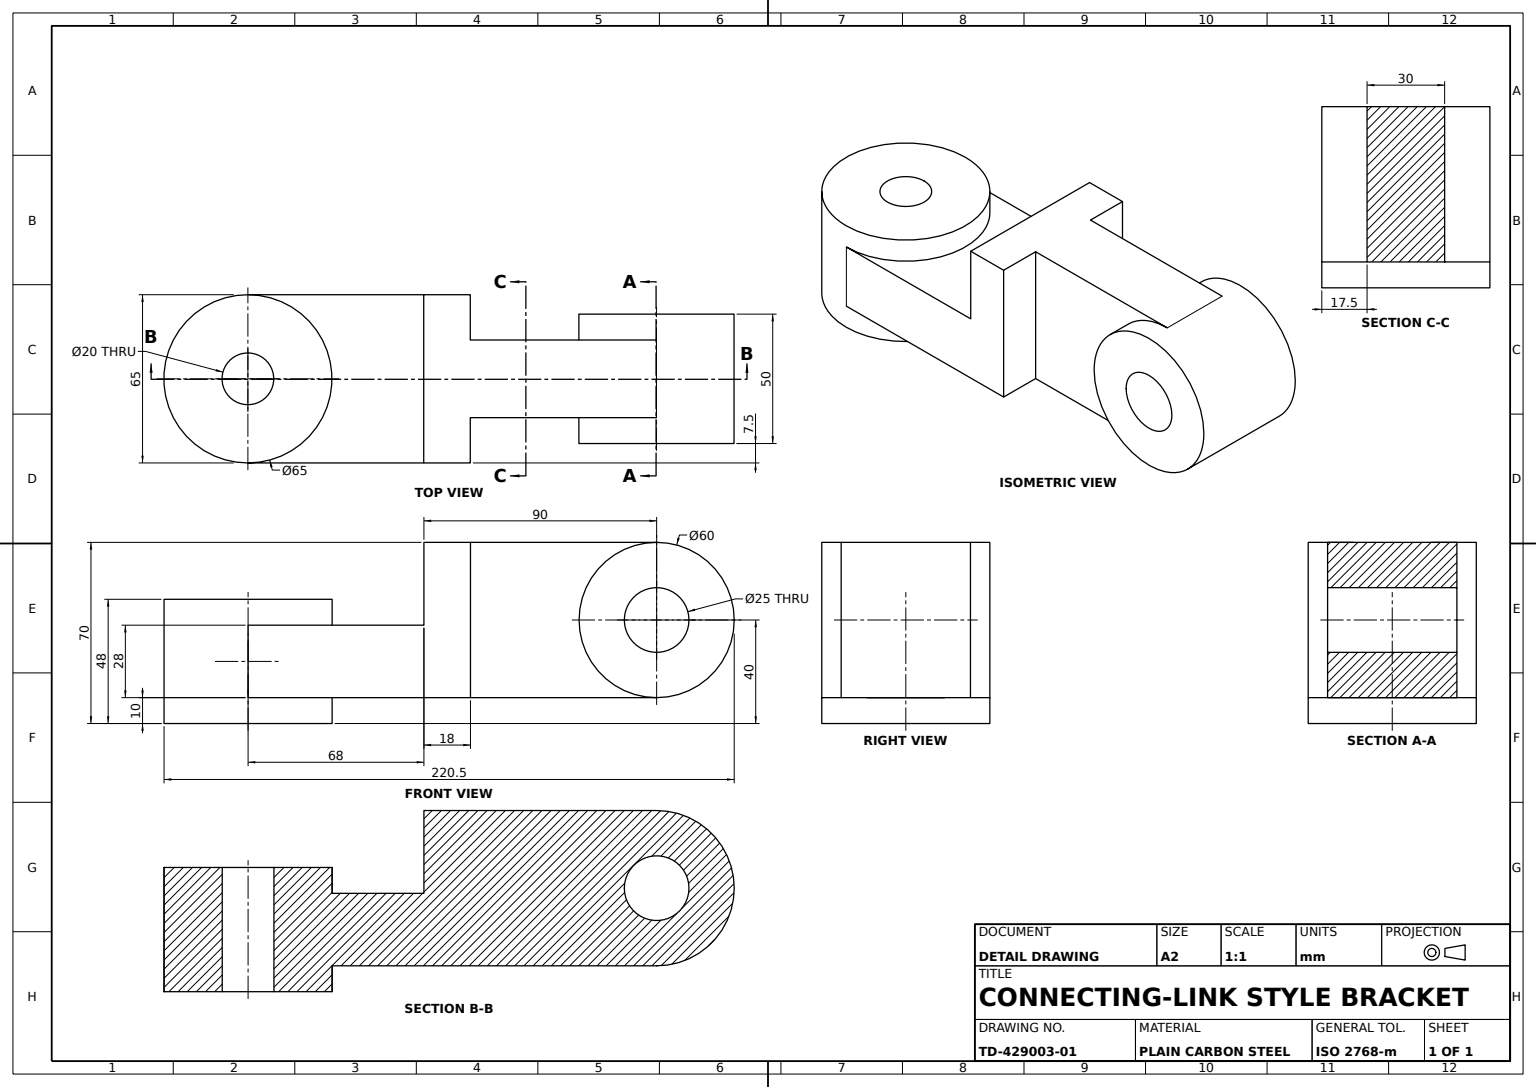
from build123d import *

# Parameters (mm, degrees)
MAIN_BODY_DEPTH                 = 65
CENTER_PAD_SKETCH_W             = 65
CENTER_PAD_SKETCH_H             = 28
CENTER_PAD_DEPTH                = 18
VERTICAL_BOSS_SKETCH_R          = 32.5
VERTICAL_BOSS_DEPTH             = 48
VERTICAL_START                  = 10
VERTICAL_BOSS_COLLAR_SKETCH_R   = 32.5
VERTICAL_BOSS_COLLAR_DEPTH      = 10
VERTICAL_START_2                = -10
VERTICAL_BOSS_RELIEF_SKETCH_R   = 32.5
VERTICAL_BOSS_RELIEF_CUT_DEPTH  = 10
VERTICAL_BORE_SKETCH_R          = 10
VERTICAL_BORE_20_DEPTH          = 48
ARM_DEPTH                       = 60
HORIZONTAL_BOSS_SKETCH_R        = 30
HORIZONTAL_BOSS_DEPTH           = 40
HORIZONTAL_START                = 10
HORIZONTAL_BOSS_COLLAR_SKETCH_R = 30
HORIZONTAL_BOSS_COLLAR_DEPTH    = 10
HORIZONTAL_BORE_SKETCH_R        = 12.5
HORIZONTAL_BORE_25_DEPTH        = 50


with BuildPart() as part:
    # Main Body Sketch → Main Body (new body)
    with BuildSketch(Plane.XY):
        Polygon((0, -28), (0, 0), (50, 0), (50, 32), (68, 32), (68, -28), align=None)
    extrude(amount=MAIN_BODY_DEPTH)

    # Center Pad Sketch → Center Pad (add)
    with BuildSketch(Plane.ZY):
        with Locations((32.5, -14)):
            Rectangle(CENTER_PAD_SKETCH_W, CENTER_PAD_SKETCH_H)
    extrude(amount=CENTER_PAD_DEPTH)

    # Vertical Boss Sketch → Vertical Boss (add)
    with BuildSketch(Plane(origin=(0, 0, 0), x_dir=(1, 0, 0), z_dir=(0, 1, 0))):
        with Locations(Location((-18, -32.5, 0), (0, 0, 270))):
            Circle(VERTICAL_BOSS_SKETCH_R)
    extrude(amount=-VERTICAL_BOSS_DEPTH)

    # Vertical Boss Collar Sketch → Vertical Boss Collar (add)
    with BuildSketch(Plane(origin=(0, 0, 0), x_dir=(1, 0, 0), z_dir=(0, 1, 0)).offset(VERTICAL_START)):
        with Locations(Location((-18, -32.5, 0), (0, 0, 270))):
            Circle(VERTICAL_BOSS_COLLAR_SKETCH_R)
    extrude(amount=-VERTICAL_BOSS_COLLAR_DEPTH)

    # Vertical Boss Relief Sketch → Vertical Boss Relief Cut (cut)
    with BuildSketch(Plane.XZ.offset(48).offset(VERTICAL_START_2)):
        with Locations(Location((-18, 32.5, 0), (0, 0, 90))):
            Circle(VERTICAL_BOSS_RELIEF_SKETCH_R)
    extrude(amount=VERTICAL_BOSS_RELIEF_CUT_DEPTH, mode=Mode.SUBTRACT)

    # Vertical Bore Sketch → Vertical Bore Ø20 (cut)
    with BuildSketch(Plane(origin=(0, 10, 0), x_dir=(1, 0, 0), z_dir=(0, 1, 0))):
        with Locations(Location((-18, -32.5, 0), (0, 0, 270))):
            Circle(VERTICAL_BORE_SKETCH_R)
    extrude(amount=-VERTICAL_BORE_20_DEPTH, mode=Mode.SUBTRACT)

    # Arm Sketch → Arm (add)
    with BuildSketch(Plane(origin=(0, 32, 0), x_dir=(1, 0, 0), z_dir=(0, 1, 0))):
        Polygon((140, -32.5), (140, -17.5), (68, -17.5), (68, -47.5), (140, -47.5), align=None)
    extrude(amount=-ARM_DEPTH)

    # Horizontal Boss Sketch → Horizontal Boss (add)
    with BuildSketch(Plane.XY.offset(47.5)):
        with Locations((140, 2)):
            Circle(HORIZONTAL_BOSS_SKETCH_R)
    extrude(amount=-HORIZONTAL_BOSS_DEPTH)

    # Horizontal Boss Collar Sketch → Horizontal Boss Collar (add)
    with BuildSketch(Plane.XY.offset(47.5).offset(HORIZONTAL_START)):
        with Locations((140, 2)):
            Circle(HORIZONTAL_BOSS_COLLAR_SKETCH_R)
    extrude(amount=-HORIZONTAL_BOSS_COLLAR_DEPTH)

    # Horizontal Bore Sketch → Horizontal Bore Ø25 (cut)
    with BuildSketch(Plane.XY.offset(57.5)):
        with Locations((140, 2)):
            Circle(HORIZONTAL_BORE_SKETCH_R)
    extrude(amount=-HORIZONTAL_BORE_25_DEPTH, mode=Mode.SUBTRACT)


solid = part.part
